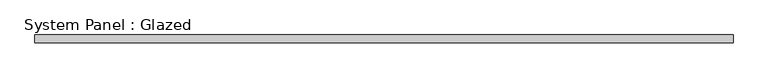
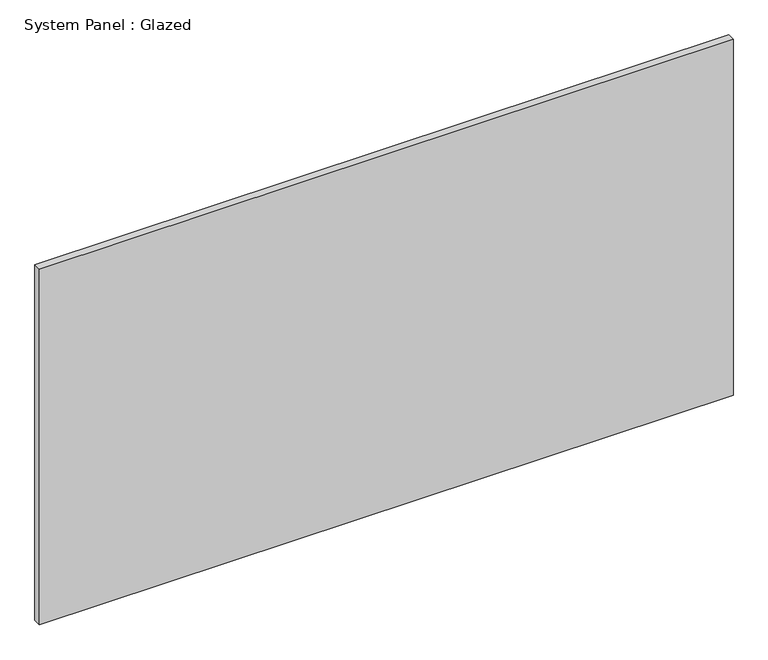
"""IFC4 building model written with IfcOpenShell, lengths in millimetres: plate geometry, System Panel : Glazed."""

from ifc_helpers import new_model, si_unit, origin, origin_with_axes, place, context, project, spatial, polyline, outline, extrude, source, transform, mapped, element, save


def system_panel_glazed_bf88fd99(model_context):
    return source(origin(), model_context, "Body", "SweptSolid", [
        extrude(outline(polyline([(1123.95, 19.05), (-1123.95, 19.05), (-1123.95, 44.45), (1123.95, 44.45), (1123.95, 19.05)])), origin_with_axes(), (0.0, 0.0, 1.0), 1219.2),
    ])


if __name__ == "__main__":
    model = new_model("IFC4")
    model_context = context("Model", 3, world=origin())
    ifc_project = project(units=[si_unit("LENGTHUNIT", "METRE", prefix="MILLI")], contexts=[model_context])
    site = spatial("IfcSite", under=ifc_project)
    building = spatial("IfcBuilding", under=site)
    placement = place(None, origin())
    system_panel_glazed_shape = system_panel_glazed_bf88fd99(model_context)
    element("IfcPlate", 1, ObjectType="System Panel : Glazed", at=placement, inside=building, context=model_context, shape_type="MappedRepresentation", body=[
        mapped(system_panel_glazed_shape, transform((0.0, 0.0, 0.0), x_axis=(1.0, 0.0, 0.0), y_axis=(0.0, 1.0, 0.0), z_axis=(0.0, 0.0, 1.0))),
    ])
    save(model, "model.ifc")

# Revit data of these elements
# Type "System Panel : Glazed"
#   Construction Type Id = "GSP4R"
#   Analytic Construction = "1/8 in Pilkington single glazing"
#   Visual Light Transmittance = 0.9
#   Solar Heat Gain Coefficient = 0.86
#   Heat Transfer Coefficient (U) = 1.18115 BTU/(h·ft²·°F)
#   Define Thermal Properties by = 1
# Element 1 (IfcPlate, "System Panel : Glazed")
#   Materials on its faces: "Glass"
# Materials
#   "Glass": class "Glass", colour RGB 0 128 192, transparency 0.75, Description = "Soda Lime Glass", Cost = 0
